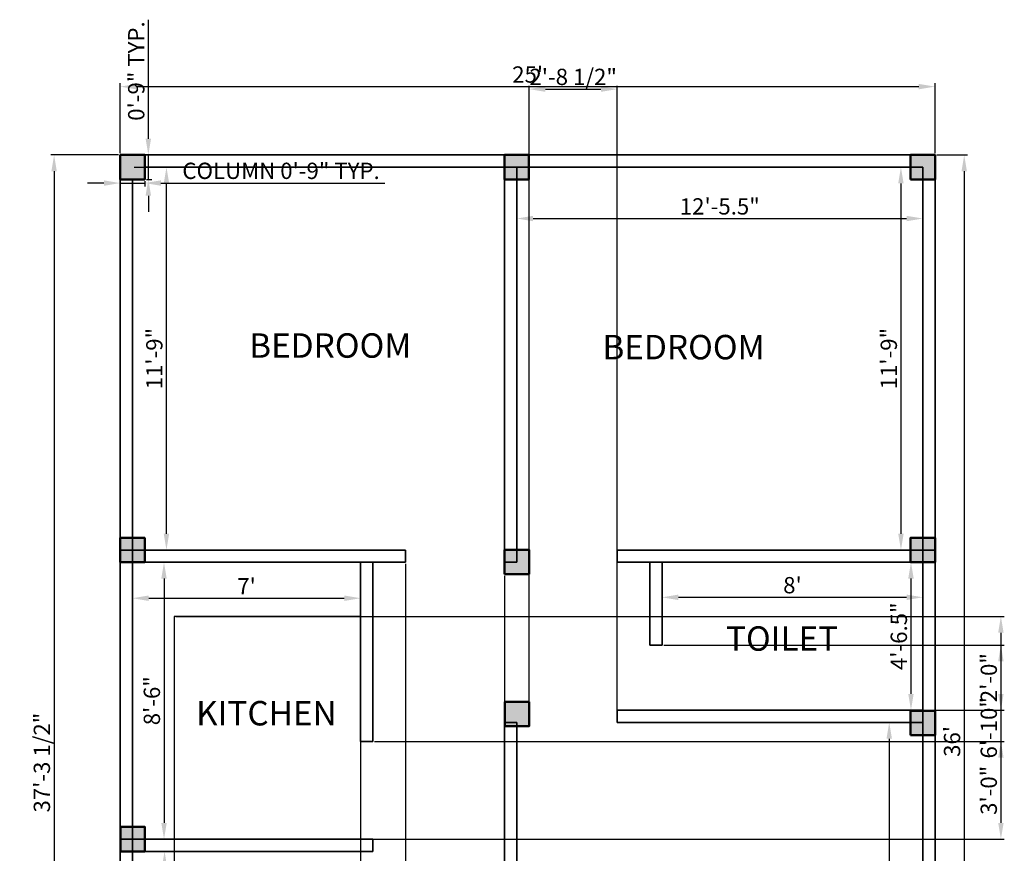
# Model space of a CAD drawing. Units: inches. Extents: x 6892 to 7255, y 6029 to 6556.
# Tile 2 of 2: x 6892 to 7255, y 6249 to 6556. Entities that reach past the tile are written whole.
import ezdxf

# ---------------------------------------------------------------- set-up
doc = ezdxf.new("R2010")
doc.units = ezdxf.units.IN
for name, color, linetype, lineweight in [('A-ANNO-DIMS', 2, 'Continuous', 18), ('A-AREA-IDEN', 7, 'Continuous', 25), ('A-COLS', 7, 'Continuous', 50), ('A-COLS-PATT', 1, 'Continuous', 13), ('A-FLOR-FIXT', 8, 'Continuous', 25), ('A-WALL', 7, 'Continuous', 35)]:
    doc.layers.add(name, color=color, linetype=linetype, lineweight=lineweight)
doc.styles.get("Standard").update_dxf_attribs({"font": 'arial.ttf'})
doc.dimstyles.new('ISO-25', dxfattribs={"dimtxt": 6, "dimasz": 6, "dimexe": 1.25, "dimexo": 0.625, "dimtad": 1, "dimlunit": 3, "dimtxsty": 'Standard', "dimcen": 2.5, "dimadec": 0, "dimazin": 0, "dimtfac": 1, "dimtmove": 0, "dimatfit": 3, "dimfxl": 1, "dimarcsym": 0})

# ---------------------------------------------------------------- blocks, each defined once
blk = doc.blocks.new('*D1')
at = {"layer": 'A-ANNO-DIMS', "color": 0, "lineweight": -2, "transparency": 16777216}
for p, q in [((6945.77, 6249.77), (6946.64, 6249.77)), ((6945.39, 6084.77), (6945.39, 6243.77)), ((6945.77, 6078.77), (6946.64, 6078.77))]:
    blk.add_line(p, q, dxfattribs=at)
at = {"layer": 'A-ANNO-DIMS', "color": 0, "transparency": 16777216}
for points in [[(6944.39, 6243.77), (6946.39, 6243.77), (6945.39, 6249.77)], [(6944.39, 6084.77), (6946.39, 6084.77), (6945.39, 6078.77)]]:
    blk.add_solid(points, dxfattribs=at)
at = {"layer": 'Defpoints', "color": 0, "transparency": 16777216}
for p in [(6945.15, 6249.77), (6945.39, 6249.77), (6945.15, 6078.77)]:
    blk.add_point(p, dxfattribs=at)
at = {"layer": 'A-ANNO-DIMS', "color": 0, "transparency": 16777216, "insert": (6941.7, 6164.27), "char_height": 6, "attachment_point": 5, "rotation": 90}
blk.add_mtext('14\'-3"', dxfattribs=at)
blk = doc.blocks.new('*D3')
at = {"layer": 'A-ANNO-DIMS', "color": 0, "lineweight": -2, "transparency": 16777216}
for p, q in [((6933.57, 6355.65), (6933.57, 6341.77)), ((7017.57, 6355.65), (7017.57, 6341.77)), ((6939.57, 6343.02), (7011.57, 6343.02))]:
    blk.add_line(p, q, dxfattribs=at)
at = {"layer": 'A-ANNO-DIMS', "color": 0, "transparency": 16777216}
for points in [[(6939.57, 6344.02), (6939.57, 6342.02), (6933.57, 6343.02)], [(7011.57, 6344.02), (7011.57, 6342.02), (7017.57, 6343.02)]]:
    blk.add_solid(points, dxfattribs=at)
at = {"layer": 'Defpoints', "color": 0, "transparency": 16777216}
for p in [(6933.57, 6356.27), (7017.57, 6356.27), (7017.57, 6343.02)]:
    blk.add_point(p, dxfattribs=at)
at = {"layer": 'A-ANNO-DIMS', "color": 0, "transparency": 16777216, "insert": (6975.57, 6346.64), "char_height": 6, "attachment_point": 5}
blk.add_mtext("7'", dxfattribs=at)
blk = doc.blocks.new('*D4')
at = {"layer": 'A-ANNO-DIMS', "color": 0, "lineweight": -2, "transparency": 16777216}
for p, q in [((6934.2, 6356.27), (6946.44, 6356.27)), ((6945.19, 6350.27), (6945.19, 6260.27)), ((6934.2, 6254.27), (6946.44, 6254.27))]:
    blk.add_line(p, q, dxfattribs=at)
at = {"layer": 'A-ANNO-DIMS', "color": 0, "transparency": 16777216}
for points in [[(6944.19, 6350.27), (6946.19, 6350.27), (6945.19, 6356.27)], [(6944.19, 6260.27), (6946.19, 6260.27), (6945.19, 6254.27)]]:
    blk.add_solid(points, dxfattribs=at)
at = {"layer": 'Defpoints', "color": 0, "transparency": 16777216}
for p in [(6933.57, 6356.27), (6933.57, 6254.27), (6945.19, 6254.27)]:
    blk.add_point(p, dxfattribs=at)
at = {"layer": 'A-ANNO-DIMS', "color": 0, "transparency": 16777216, "insert": (6941.5, 6305.27), "char_height": 6, "attachment_point": 5, "rotation": 90}
blk.add_mtext('8\'-6"', dxfattribs=at)
blk = doc.blocks.new('*D5')
at = {"layer": 'A-ANNO-DIMS', "color": 0, "lineweight": -2, "transparency": 16777216}
for p, q in [((6934.2, 6501.77), (6947.34, 6501.77)), ((6946.09, 6366.77), (6946.09, 6495.77)), ((6934.2, 6360.77), (6947.34, 6360.77))]:
    blk.add_line(p, q, dxfattribs=at)
at = {"layer": 'A-ANNO-DIMS', "color": 0, "transparency": 16777216}
for points in [[(6945.09, 6495.77), (6947.09, 6495.77), (6946.09, 6501.77)], [(6945.09, 6366.77), (6947.09, 6366.77), (6946.09, 6360.77)]]:
    blk.add_solid(points, dxfattribs=at)
at = {"layer": 'Defpoints', "color": 0, "transparency": 16777216}
for p in [(6933.57, 6501.77), (6946.09, 6501.77), (6933.57, 6360.77)]:
    blk.add_point(p, dxfattribs=at)
at = {"layer": 'A-ANNO-DIMS', "color": 0, "transparency": 16777216, "insert": (6942.4, 6431.27), "char_height": 6, "attachment_point": 5, "rotation": 90}
blk.add_mtext('11\'-9"', dxfattribs=at)
blk = doc.blocks.new('*D6')
at = {"layer": 'A-ANNO-DIMS', "color": 0, "lineweight": -2, "transparency": 16777216}
for p, q in [((7075.07, 6501.15), (7075.07, 6481.61)), ((7224.57, 6501.15), (7224.57, 6481.61)), ((7081.07, 6482.86), (7218.57, 6482.86))]:
    blk.add_line(p, q, dxfattribs=at)
at = {"layer": 'A-ANNO-DIMS', "color": 0, "transparency": 16777216}
for points in [[(7081.07, 6483.86), (7081.07, 6481.86), (7075.07, 6482.86)], [(7218.57, 6483.86), (7218.57, 6481.86), (7224.57, 6482.86)]]:
    blk.add_solid(points, dxfattribs=at)
at = {"layer": 'Defpoints', "color": 0, "transparency": 16777216}
for p in [(7075.07, 6501.77), (7224.57, 6501.77), (7224.57, 6482.86)]:
    blk.add_point(p, dxfattribs=at)
at = {"layer": 'A-ANNO-DIMS', "color": 0, "transparency": 16777216, "insert": (7149.82, 6486.55), "char_height": 6, "attachment_point": 5}
blk.add_mtext('12\'-5.5"', dxfattribs=at)
blk = doc.blocks.new('*D7')
at = {"layer": 'A-ANNO-DIMS', "color": 0, "lineweight": -2, "transparency": 16777216}
for p, q in [((7223.95, 6501.77), (7215.26, 6501.77)), ((7216.51, 6495.77), (7216.51, 6366.77)), ((7223.95, 6360.77), (7215.26, 6360.77))]:
    blk.add_line(p, q, dxfattribs=at)
at = {"layer": 'A-ANNO-DIMS', "color": 0, "transparency": 16777216}
for points in [[(7215.51, 6495.77), (7217.51, 6495.77), (7216.51, 6501.77)], [(7215.51, 6366.77), (7217.51, 6366.77), (7216.51, 6360.77)]]:
    blk.add_solid(points, dxfattribs=at)
at = {"layer": 'Defpoints', "color": 0, "transparency": 16777216}
for p in [(7224.57, 6501.77), (7216.51, 6360.77), (7224.57, 6360.77)]:
    blk.add_point(p, dxfattribs=at)
at = {"layer": 'A-ANNO-DIMS', "color": 0, "transparency": 16777216, "insert": (7212.82, 6431.27), "char_height": 6, "attachment_point": 5, "rotation": 90}
blk.add_mtext('11\'-9"', dxfattribs=at)
blk = doc.blocks.new('*D8')
at = {"layer": 'A-ANNO-DIMS', "color": 0, "lineweight": -2, "transparency": 16777216}
for p, q in [((7128.57, 6355.65), (7128.57, 6342.1)), ((7224.57, 6355.65), (7224.57, 6342.1)), ((7134.57, 6343.35), (7218.57, 6343.35))]:
    blk.add_line(p, q, dxfattribs=at)
at = {"layer": 'A-ANNO-DIMS', "color": 0, "transparency": 16777216}
for points in [[(7134.57, 6344.35), (7134.57, 6342.35), (7128.57, 6343.35)], [(7218.57, 6344.35), (7218.57, 6342.35), (7224.57, 6343.35)]]:
    blk.add_solid(points, dxfattribs=at)
at = {"layer": 'Defpoints', "color": 0, "transparency": 16777216}
for p in [(7128.57, 6356.27), (7224.57, 6356.27), (7224.57, 6343.35)]:
    blk.add_point(p, dxfattribs=at)
at = {"layer": 'A-ANNO-DIMS', "color": 0, "transparency": 16777216, "insert": (7176.57, 6347.04), "char_height": 6, "attachment_point": 5}
blk.add_mtext("8'", dxfattribs=at)
blk = doc.blocks.new('*D9')
at = {"layer": 'A-ANNO-DIMS', "color": 0, "lineweight": -2, "transparency": 16777216}
for p, q in [((7223.95, 6356.27), (7218.96, 6356.27)), ((7220.21, 6350.27), (7220.21, 6307.77)), ((7223.95, 6301.77), (7218.96, 6301.77))]:
    blk.add_line(p, q, dxfattribs=at)
at = {"layer": 'A-ANNO-DIMS', "color": 0, "transparency": 16777216}
for points in [[(7219.21, 6350.27), (7221.21, 6350.27), (7220.21, 6356.27)], [(7219.21, 6307.77), (7221.21, 6307.77), (7220.21, 6301.77)]]:
    blk.add_solid(points, dxfattribs=at)
at = {"layer": 'Defpoints', "color": 0, "transparency": 16777216}
for p in [(7224.57, 6356.27), (7220.21, 6301.77), (7224.57, 6301.77)]:
    blk.add_point(p, dxfattribs=at)
at = {"layer": 'A-ANNO-DIMS', "color": 0, "transparency": 16777216, "insert": (7216.52, 6329.02), "char_height": 6, "attachment_point": 5, "rotation": 90}
blk.add_mtext('4\'-6.5"', dxfattribs=at)
blk = doc.blocks.new('*D11')
at = {"layer": 'A-ANNO-DIMS', "color": 0, "lineweight": -2, "transparency": 16777216}
for p, q in [((7223.95, 6297.27), (7210.95, 6297.27)), ((7212.2, 6291.27), (7212.2, 6167.27)), ((7223.95, 6161.27), (7210.95, 6161.27))]:
    blk.add_line(p, q, dxfattribs=at)
at = {"layer": 'A-ANNO-DIMS', "color": 0, "transparency": 16777216}
for points in [[(7211.2, 6291.27), (7213.2, 6291.27), (7212.2, 6297.27)], [(7211.2, 6167.27), (7213.2, 6167.27), (7212.2, 6161.27)]]:
    blk.add_solid(points, dxfattribs=at)
at = {"layer": 'Defpoints', "color": 0, "transparency": 16777216}
for p in [(7224.57, 6297.27), (7212.2, 6161.27), (7224.57, 6161.27)]:
    blk.add_point(p, dxfattribs=at)
at = {"layer": 'A-ANNO-DIMS', "color": 0, "transparency": 16777216, "insert": (7208.56, 6229.27), "char_height": 6, "attachment_point": 5, "rotation": 90}
blk.add_mtext('11\'-4"', dxfattribs=at)
blk = doc.blocks.new('*D15')
at = {"layer": 'A-ANNO-DIMS', "color": 0, "lineweight": -2, "transparency": 16777216}
for p, q in [((6929.07, 6506.9), (6929.07, 6532.69)), ((7229.07, 6506.9), (7229.07, 6532.69)), ((6935.07, 6531.44), (7223.07, 6531.44))]:
    blk.add_line(p, q, dxfattribs=at)
at = {"layer": 'A-ANNO-DIMS', "color": 0, "transparency": 16777216}
for points in [[(6935.07, 6532.44), (6935.07, 6530.44), (6929.07, 6531.44)], [(7223.07, 6532.44), (7223.07, 6530.44), (7229.07, 6531.44)]]:
    blk.add_solid(points, dxfattribs=at)
at = {"layer": 'Defpoints', "color": 0, "transparency": 16777216}
for p in [(7229.07, 6531.44), (6929.07, 6506.27), (7229.07, 6506.27)]:
    blk.add_point(p, dxfattribs=at)
at = {"layer": 'A-ANNO-DIMS', "color": 0, "transparency": 16777216, "insert": (7079.07, 6535.12), "char_height": 6, "attachment_point": 5}
blk.add_mtext("25'", dxfattribs=at)
blk = doc.blocks.new('*D16')
at = {"layer": 'A-ANNO-DIMS', "color": 0, "lineweight": -2, "transparency": 16777216}
for p, q in [((7229.7, 6506.27), (7241.06, 6506.27)), ((7239.81, 6500.27), (7239.81, 6080.27)), ((7229.7, 6074.27), (7241.06, 6074.27))]:
    blk.add_line(p, q, dxfattribs=at)
at = {"layer": 'A-ANNO-DIMS', "color": 0, "transparency": 16777216}
for points in [[(7238.81, 6500.27), (7240.81, 6500.27), (7239.81, 6506.27)], [(7238.81, 6080.27), (7240.81, 6080.27), (7239.81, 6074.27)]]:
    blk.add_solid(points, dxfattribs=at)
at = {"layer": 'Defpoints', "color": 0, "transparency": 16777216}
for p in [(7229.07, 6506.27), (7229.07, 6074.27), (7239.81, 6074.27)]:
    blk.add_point(p, dxfattribs=at)
at = {"layer": 'A-ANNO-DIMS', "color": 0, "transparency": 16777216, "insert": (7236.12, 6290.27), "char_height": 6, "attachment_point": 5, "rotation": 90}
blk.add_mtext("36'", dxfattribs=at)
blk = doc.blocks.new('COL-9IN-SQ')
blk.add_lwpolyline([(0, 0), (9, 0), (9, 9), (0, 9)], close=True)
blk = doc.blocks.new('*D18')
at = {"layer": 'A-ANNO-DIMS', "color": 0, "lineweight": -2, "transparency": 16777216}
for p, q in [((6929.07, 6496.65), (6929.07, 6494.67)), ((6938.07, 6496.65), (6938.07, 6494.67)), ((6923.07, 6495.92), (6917.07, 6495.92)), ((6929.07, 6495.92), (6938.07, 6495.92)), ((6944.07, 6495.92), (7026.48, 6495.92))]:
    blk.add_line(p, q, dxfattribs=at)
at = {"layer": 'A-ANNO-DIMS', "color": 0, "transparency": 16777216}
for points in [[(6923.07, 6496.92), (6923.07, 6494.92), (6929.07, 6495.92)], [(6944.07, 6496.92), (6944.07, 6494.92), (6938.07, 6495.92)]]:
    blk.add_solid(points, dxfattribs=at)
at = {"layer": 'Defpoints', "color": 0, "transparency": 16777216}
for p in [(6929.07, 6497.27), (6938.07, 6497.27), (6938.07, 6495.92)]:
    blk.add_point(p, dxfattribs=at)
at = {"layer": 'A-ANNO-DIMS', "color": 0, "transparency": 16777216, "insert": (6988.28, 6499.65), "char_height": 6, "attachment_point": 5}
blk.add_mtext('COLUMN 0\'-9" TYP.', dxfattribs=at)
blk = doc.blocks.new('*D19')
at = {"layer": 'A-ANNO-DIMS', "color": 0, "lineweight": -2, "transparency": 16777216}
for p, q in [((6939.42, 6512.27), (6939.42, 6556.09)), ((6938.7, 6506.27), (6940.67, 6506.27)), ((6939.42, 6497.27), (6939.42, 6506.27)), ((6938.7, 6497.27), (6940.67, 6497.27)), ((6939.42, 6491.27), (6939.42, 6485.27))]:
    blk.add_line(p, q, dxfattribs=at)
at = {"layer": 'A-ANNO-DIMS', "color": 0, "transparency": 16777216}
for points in [[(6938.42, 6512.27), (6940.42, 6512.27), (6939.42, 6506.27)], [(6938.42, 6491.27), (6940.42, 6491.27), (6939.42, 6497.27)]]:
    blk.add_solid(points, dxfattribs=at)
at = {"layer": 'Defpoints', "color": 0, "transparency": 16777216}
for p in [(6938.07, 6506.27), (6939.42, 6506.27), (6938.07, 6497.27)]:
    blk.add_point(p, dxfattribs=at)
at = {"layer": 'A-ANNO-DIMS', "color": 0, "transparency": 16777216, "insert": (6935.74, 6537.18), "char_height": 6, "attachment_point": 5, "rotation": 90}
blk.add_mtext('0\'-9" TYP.', dxfattribs=at)
blk = doc.blocks.new('*D20')
at = {"layer": 'A-ANNO-DIMS', "color": 0, "lineweight": -2, "transparency": 16777216}
for p, q in [((6928.45, 6506.27), (6903.48, 6506.27)), ((6904.73, 6500.27), (6904.73, 6064.66)), ((7017.45, 6058.66), (6903.48, 6058.66))]:
    blk.add_line(p, q, dxfattribs=at)
at = {"layer": 'A-ANNO-DIMS', "color": 0, "transparency": 16777216}
for points in [[(6903.73, 6500.27), (6905.73, 6500.27), (6904.73, 6506.27)], [(6903.73, 6064.66), (6905.73, 6064.66), (6904.73, 6058.66)]]:
    blk.add_solid(points, dxfattribs=at)
at = {"layer": 'Defpoints', "color": 0, "transparency": 16777216}
for p in [(6929.07, 6506.27), (6904.73, 6058.66), (7018.07, 6058.66)]:
    blk.add_point(p, dxfattribs=at)
at = {"layer": 'A-ANNO-DIMS', "color": 0, "transparency": 16777216, "insert": (6901, 6282.47), "char_height": 6, "attachment_point": 5, "rotation": 90}
blk.add_mtext('37\'-3 1/2"', dxfattribs=at)
blk = doc.blocks.new('*D22')
at = {"layer": 'A-ANNO-DIMS', "color": 0, "lineweight": -2, "transparency": 16777216}
for p, q in [((7034.07, 6355.65), (7034.07, 6033.16)), ((7070.6, 6351.27), (7070.6, 6033.16)), ((7040.07, 6034.41), (7064.6, 6034.41))]:
    blk.add_line(p, q, dxfattribs=at)
at = {"layer": 'A-ANNO-DIMS', "color": 0, "transparency": 16777216}
for points in [[(7040.07, 6035.41), (7040.07, 6033.41), (7034.07, 6034.41)], [(7064.6, 6035.41), (7064.6, 6033.41), (7070.6, 6034.41)]]:
    blk.add_solid(points, dxfattribs=at)
at = {"layer": 'Defpoints', "color": 0, "transparency": 16777216}
for p in [(7034.07, 6356.27), (7070.6, 6351.9), (7070.6, 6034.41)]:
    blk.add_point(p, dxfattribs=at)
at = {"layer": 'A-ANNO-DIMS', "color": 0, "transparency": 16777216, "insert": (7052.34, 6038.14), "char_height": 6, "attachment_point": 5}
blk.add_mtext('3\'-0 1/2"', dxfattribs=at)
blk = doc.blocks.new('*D23')
at = {"layer": 'A-ANNO-DIMS', "color": 0, "lineweight": -2, "transparency": 16777216}
for p, q in [((7079.6, 6361.52), (7079.6, 6531.77)), ((7085.6, 6530.52), (7106.07, 6530.52)), ((7112.07, 6361.4), (7112.07, 6531.77))]:
    blk.add_line(p, q, dxfattribs=at)
at = {"layer": 'A-ANNO-DIMS', "color": 0, "transparency": 16777216}
for points in [[(7085.6, 6531.52), (7085.6, 6529.52), (7079.6, 6530.52)], [(7106.07, 6531.52), (7106.07, 6529.52), (7112.07, 6530.52)]]:
    blk.add_solid(points, dxfattribs=at)
at = {"layer": 'Defpoints', "color": 0, "transparency": 16777216}
for p in [(7112.07, 6530.52), (7079.6, 6360.9), (7112.07, 6360.77)]:
    blk.add_point(p, dxfattribs=at)
at = {"layer": 'A-ANNO-DIMS', "color": 0, "transparency": 16777216, "insert": (7095.84, 6534.25), "char_height": 6, "attachment_point": 5}
blk.add_mtext('2\'-8 1/2"', dxfattribs=at)
blk = doc.blocks.new('*D24')
at = {"layer": 'A-ANNO-DIMS', "color": 0, "lineweight": -2, "transparency": 16777216}
for p, q in [((7022.7, 6290.27), (7254.57, 6290.27)), ((7253.32, 6284.27), (7253.32, 6260.27)), ((7022.7, 6254.27), (7254.57, 6254.27))]:
    blk.add_line(p, q, dxfattribs=at)
at = {"layer": 'A-ANNO-DIMS', "color": 0, "transparency": 16777216}
for points in [[(7252.32, 6284.27), (7254.32, 6284.27), (7253.32, 6290.27)], [(7252.32, 6260.27), (7254.32, 6260.27), (7253.32, 6254.27)]]:
    blk.add_solid(points, dxfattribs=at)
at = {"layer": 'Defpoints', "color": 0, "transparency": 16777216}
for p in [(7022.07, 6290.27), (7022.07, 6254.27), (7253.32, 6254.27)]:
    blk.add_point(p, dxfattribs=at)
at = {"layer": 'A-ANNO-DIMS', "color": 0, "transparency": 16777216, "insert": (7249.63, 6272.27), "char_height": 6, "attachment_point": 5, "rotation": 90}
blk.add_mtext('3\'-0"', dxfattribs=at)
blk = doc.blocks.new('*D25')
at = {"layer": 'A-ANNO-DIMS', "color": 0, "lineweight": -2, "transparency": 16777216}
for p, q in [((7129.2, 6325.77), (7254.57, 6325.77)), ((7253.32, 6319.77), (7253.32, 6307.77)), ((7112.7, 6301.77), (7254.57, 6301.77))]:
    blk.add_line(p, q, dxfattribs=at)
at = {"layer": 'A-ANNO-DIMS', "color": 0, "transparency": 16777216}
for points in [[(7252.32, 6319.77), (7254.32, 6319.77), (7253.32, 6325.77)], [(7252.32, 6307.77), (7254.32, 6307.77), (7253.32, 6301.77)]]:
    blk.add_solid(points, dxfattribs=at)
at = {"layer": 'Defpoints', "color": 0, "transparency": 16777216}
for p in [(7128.57, 6325.77), (7112.07, 6301.77), (7253.32, 6301.77)]:
    blk.add_point(p, dxfattribs=at)
at = {"layer": 'A-ANNO-DIMS', "color": 0, "transparency": 16777216, "insert": (7249.64, 6313.77), "char_height": 6, "attachment_point": 5, "rotation": 90}
blk.add_mtext('2\'-0"', dxfattribs=at)
blk = doc.blocks.new('*D26')
at = {"layer": 'A-ANNO-DIMS', "color": 0, "lineweight": -2, "transparency": 16777216}
for p, q in [((7079.63, 6296.47), (7079.63, 6531.77)), ((7085.63, 6530.52), (7106.07, 6530.52)), ((7112.07, 6297.9), (7112.07, 6531.77))]:
    blk.add_line(p, q, dxfattribs=at)
at = {"layer": 'A-ANNO-DIMS', "color": 0, "transparency": 16777216}
for points in [[(7085.63, 6531.52), (7085.63, 6529.52), (7079.63, 6530.52)], [(7106.07, 6531.52), (7106.07, 6529.52), (7112.07, 6530.52)]]:
    blk.add_solid(points, dxfattribs=at)
at = {"layer": 'Defpoints', "color": 0, "transparency": 16777216}
for p in [(7112.07, 6530.52), (7112.07, 6297.27), (7079.63, 6295.85)]:
    blk.add_point(p, dxfattribs=at)
at = {"layer": 'A-ANNO-DIMS', "color": 0, "transparency": 16777216, "insert": (7095.85, 6534.25), "char_height": 6, "attachment_point": 5}
blk.add_mtext('2\'-8 1/2"', dxfattribs=at)
blk = doc.blocks.new('*D28')
at = {"layer": 'A-ANNO-DIMS', "color": 0, "lineweight": -2, "transparency": 16777216}
for p, q in [((6948.94, 6335.71), (6948.94, 6033.16)), ((7017.57, 6335.71), (7017.57, 6033.16)), ((6954.94, 6034.41), (7011.57, 6034.41))]:
    blk.add_line(p, q, dxfattribs=at)
at = {"layer": 'A-ANNO-DIMS', "color": 0, "transparency": 16777216}
for points in [[(6954.94, 6035.41), (6954.94, 6033.41), (6948.94, 6034.41)], [(7011.57, 6035.41), (7011.57, 6033.41), (7017.57, 6034.41)]]:
    blk.add_solid(points, dxfattribs=at)
at = {"layer": 'Defpoints', "color": 0, "transparency": 16777216}
for p in [(6948.94, 6336.33), (7017.57, 6336.33), (7017.57, 6034.41)]:
    blk.add_point(p, dxfattribs=at)
at = {"layer": 'A-ANNO-DIMS', "color": 0, "transparency": 16777216, "insert": (6983.26, 6038.14), "char_height": 6, "attachment_point": 5}
blk.add_mtext('5\'-8 1/2"', dxfattribs=at)
blk = doc.blocks.new('*D29')
at = {"layer": 'A-ANNO-DIMS', "color": 0, "lineweight": -2, "transparency": 16777216}
for p, q in [((6949.57, 6336.33), (7254.57, 6336.33)), ((7253.32, 6330.33), (7253.32, 6260.27)), ((6949.57, 6254.27), (7254.57, 6254.27))]:
    blk.add_line(p, q, dxfattribs=at)
at = {"layer": 'A-ANNO-DIMS', "color": 0, "transparency": 16777216}
for points in [[(7252.32, 6330.33), (7254.32, 6330.33), (7253.32, 6336.33)], [(7252.32, 6260.27), (7254.32, 6260.27), (7253.32, 6254.27)]]:
    blk.add_solid(points, dxfattribs=at)
at = {"layer": 'Defpoints', "color": 0, "transparency": 16777216}
for p in [(6948.94, 6336.33), (6948.94, 6254.27), (7253.32, 6254.27)]:
    blk.add_point(p, dxfattribs=at)
at = {"layer": 'A-ANNO-DIMS', "color": 0, "transparency": 16777216, "insert": (7249.64, 6295.3), "char_height": 6, "attachment_point": 5, "rotation": 90}
blk.add_mtext('6\'-10"', dxfattribs=at)

msp = doc.modelspace()

# ---------------------------------------------------------------- hatches: boundary and pattern name
at = {"layer": 'A-COLS-PATT'}
h = msp.add_hatch(color=256, dxfattribs=at)
h.dxf.hatch_style = 1
h.paths.add_polyline_path([(6938.074, 6506.271), (6929.074, 6506.271), (6929.074, 6497.271), (6938.074, 6497.271)])
h.paths.add_polyline_path([(7079.574, 6506.271), (7070.574, 6506.271), (7070.574, 6501.771), (7079.574, 6501.771)])
h.paths.add_polyline_path([(7079.574, 6501.771), (7075.074, 6501.771), (7075.074, 6497.271), (7079.574, 6497.271)])
h.paths.add_polyline_path([(7075.074, 6501.771), (7070.574, 6501.771), (7070.574, 6497.271), (7075.074, 6497.271)])
h.paths.add_polyline_path([(7229.074, 6506.271), (7220.074, 6506.271), (7220.074, 6501.771), (7224.574, 6501.771), (7224.574, 6497.271), (7229.074, 6497.271)])
h.paths.add_polyline_path([(7224.574, 6501.771), (7220.074, 6501.771), (7220.074, 6497.271), (7224.574, 6497.271)], flags=17)
h.paths.add_polyline_path([(7224.574, 6365.271), (7220.074, 6365.271), (7220.074, 6360.771), (7224.574, 6360.771)])
h.paths.add_polyline_path([(7229.074, 6365.271), (7224.574, 6365.271), (7224.574, 6360.771), (7229.074, 6360.771)])
h.paths.add_polyline_path([(7229.074, 6360.771), (7224.574, 6360.771), (7224.574, 6356.271), (7229.074, 6356.271)])
h.paths.add_polyline_path([(7224.574, 6360.771), (7220.074, 6360.771), (7220.074, 6356.271), (7224.574, 6356.271)])
h.paths.add_polyline_path([(6938.094, 6360.771), (6933.574, 6360.771), (6933.574, 6356.271), (6938.094, 6356.271)])
h.paths.add_polyline_path([(6938.094, 6365.243), (6933.574, 6365.243), (6933.574, 6360.771), (6938.094, 6360.771)])
h.paths.add_polyline_path([(6933.574, 6365.243), (6929.094, 6365.243), (6929.094, 6360.771), (6933.574, 6360.771)])
h.paths.add_polyline_path([(6933.574, 6360.771), (6929.094, 6360.771), (6929.094, 6356.271), (6933.574, 6356.271)])
h.paths.add_polyline_path([(7075.074, 6360.771), (7070.605, 6360.771), (7070.605, 6356.271), (7075.074, 6356.271)], flags=17)
h.paths.add_polyline_path([(7079.605, 6360.898), (7075.074, 6360.898), (7075.074, 6356.271), (7070.605, 6356.271), (7070.605, 6351.898), (7079.605, 6351.898)])
h.paths.add_polyline_path([(7079.634, 6304.845), (7070.634, 6304.845), (7070.634, 6297.271), (7075.074, 6297.271), (7075.074, 6295.845), (7079.634, 6295.845)])
h.paths.add_polyline_path([(7075.074, 6297.271), (7070.634, 6297.271), (7070.634, 6295.845), (7075.074, 6295.845)], flags=17)
h.paths.add_polyline_path([(6938.172, 6258.771), (6933.574, 6258.771), (6933.574, 6254.271), (6938.172, 6254.271)])
h.paths.add_polyline_path([(6933.574, 6258.771), (6929.172, 6258.771), (6929.172, 6254.271), (6933.574, 6254.271)])
h.paths.add_polyline_path([(6933.574, 6254.271), (6929.172, 6254.271), (6929.172, 6249.771), (6933.574, 6249.771)])
h.paths.add_polyline_path([(6938.172, 6254.271), (6933.574, 6254.271), (6933.574, 6249.771), (6938.172, 6249.771)])
h.paths.add_polyline_path([(7229.074, 6301.605), (7224.574, 6301.605), (7224.574, 6297.271), (7224.574, 6292.605), (7229.074, 6292.605)])
h.paths.add_polyline_path([(7224.574, 6297.271), (7220.074, 6297.271), (7220.074, 6292.605), (7224.574, 6292.605)])
h.paths.add_polyline_path([(7224.574, 6301.605), (7220.074, 6301.605), (7220.074, 6297.271), (7224.574, 6297.271)])

# ---------------------------------------------------------------- linework, layer by layer
at = {"layer": 'A-FLOR-FIXT'}
for p, q in [((7017.574, 6336.334), (6948.942, 6336.334)), ((6948.942, 6336.334), (6948.942, 6254.271))]:
    msp.add_line(p, q, dxfattribs=at)
at = {"layer": 'A-WALL'}
for p, q in [((6929.074, 6506.271), (7229.074, 6506.271)), ((6929.074, 6074.271), (6929.074, 6506.271)), ((7229.074, 6506.271), (7229.074, 6074.271)), ((6938.074, 6501.771), (7224.574, 6501.771)), ((7070.574, 6501.771), (7070.574, 6356.271)), ((7075.074, 6501.771), (7075.074, 6356.271)), ((7224.574, 6501.771), (7224.574, 6074.271)), ((6933.574, 6074.271), (6933.574, 6497.271)), ((7034.074, 6360.771), (6929.074, 6360.771)), ((7034.074, 6356.271), (7034.074, 6360.771)), ((7075.074, 6360.771), (7070.574, 6360.771)), ((7229.074, 6360.771), (7112.074, 6360.771)), ((7112.074, 6356.271), (7112.074, 6360.771)), ((7034.074, 6356.271), (6929.074, 6356.271)), ((7017.574, 6356.271), (7017.574, 6290.271)), ((7022.074, 6356.271), (7022.074, 6290.271)), ((7022.074, 6356.271), (7034.074, 6356.271)), ((7075.074, 6356.271), (7070.574, 6356.271)), ((7229.074, 6356.271), (7112.074, 6356.271)), ((7124.074, 6356.271), (7112.074, 6356.271)), ((7124.074, 6356.271), (7124.074, 6325.771)), ((7128.574, 6356.271), (7128.574, 6325.771)), ((7224.574, 6356.271), (7224.574, 6297.271)), ((7124.074, 6325.771), (7128.574, 6325.771)), ((7112.074, 6301.771), (7224.574, 6301.771)), ((7112.074, 6301.771), (7112.074, 6297.271)), ((7075.074, 6297.271), (7070.574, 6297.271)), ((7070.574, 6297.271), (7070.574, 6249.771)), ((7075.074, 6249.771), (7075.074, 6297.271)), ((7112.074, 6297.271), (7224.574, 6297.271)), ((7017.574, 6290.271), (7022.074, 6290.271)), ((7022.074, 6254.271), (6929.074, 6254.271)), ((7022.074, 6254.271), (7022.074, 6249.771)), ((7022.074, 6249.771), (6929.074, 6249.771)), ((7070.574, 6249.771), (7070.574, 6156.771)), ((7075.074, 6249.771), (7075.074, 6156.771))]:
    msp.add_line(p, q, dxfattribs=at)

# ---------------------------------------------------------------- block references
at = {"layer": 'A-COLS'}
for p in [(6929.074, 6497.271), (7070.574, 6497.271), (7220.074, 6497.271), (6929.095, 6356.243), (7220.074, 6356.271), (7070.605, 6351.897), (7070.634, 6295.845), (7220.074, 6292.604), (6929.172, 6249.771)]:
    msp.add_blockref('COL-9IN-SQ', p, dxfattribs=at)

# ---------------------------------------------------------------- texts
at = {"layer": 'A-AREA-IDEN', "char_height": 9, "attachment_point": 1}
for s, width, heights, insert in [('BEDROOM', 37.83075, [0], (6976.54, 6440.588)), ('BEDROOM', 43.8085, [0.785], (7106.616, 6439.999)), ('TOILET', 37.75614, [0], (7152.097, 6332.674)), ('KITCHEN', 42.3338, [0], (6957.012, 6305.161))]:
    msp.add_mtext_dynamic_manual_height_columns(s, width=width, gutter_width=12.5, heights=heights, dxfattribs=dict(at, insert=insert))

# ---------------------------------------------------------------- dimensions: what is measured, and where the dimension line sits
at = {"layer": 'A-ANNO-DIMS'}
dim = msp.add_linear_dim(base=(6939.424, 6506.271), p1=(6938.074, 6497.271), p2=(6938.074, 6506.271), angle=90, text='<> TYP.', dimstyle='ISO-25', override={"dimdec": 1, "dimlfac": 1, "dimrnd": 0, "dimzin": 1, "dimdsep": 46, "dimlunit": 4, "dimfrac": 2}, dxfattribs=at)
dim.commit()
dim.dimension.update_dxf_attribs({"geometry": '*D19', "text_midpoint": (6935.735, 6537.183)})
for base, p1, p2, override, picture, middle in [((7112.074, 6530.521), (7079.605, 6360.898), (7112.074, 6360.771), {"dimdec": 1, "dimlfac": 1, "dimrnd": 0, "dimzin": 1, "dimdsep": 46, "dimlunit": 4, "dimfrac": 2}, '*D23', (7095.839, 6534.249)), ((7112.074, 6530.521), (7079.634, 6295.845), (7112.074, 6297.271), {"dimdec": 1, "dimlfac": 1, "dimrnd": 0, "dimzin": 1, "dimdsep": 46, "dimlunit": 4, "dimfrac": 2}, '*D26', (7095.854, 6534.249)), ((7229.074, 6531.436), (6929.074, 6506.271), (7229.074, 6506.271), {"dimclrd": 0, "dimclre": 0, "dimclrt": 0}, '*D15', (7079.074, 6535.125)), ((7224.574, 6482.864), (7075.074, 6501.771), (7224.574, 6501.771), {"dimclrd": 0, "dimclre": 0, "dimclrt": 0}, '*D6', (7149.824, 6486.553)), ((7017.574, 6343.019), (6933.574, 6356.271), (7017.574, 6356.271), {"dimclrd": 0, "dimclre": 0, "dimclrt": 0}, '*D3', (6975.574, 6346.644)), ((7070.605, 6034.411), (7034.074, 6356.271), (7070.605, 6351.898), {"dimdec": 1, "dimlfac": 1, "dimrnd": 0, "dimzin": 1, "dimdsep": 46, "dimlunit": 4, "dimfrac": 2}, '*D22', (7052.339, 6038.14)), ((7224.574, 6343.349), (7128.574, 6356.271), (7224.574, 6356.271), {"dimclrd": 0, "dimclre": 0, "dimclrt": 0}, '*D8', (7176.574, 6347.038)), ((7017.574, 6034.411), (6948.942, 6336.334), (7017.574, 6336.334), {"dimdec": 1, "dimlfac": 1, "dimrnd": 0, "dimzin": 1, "dimdsep": 46, "dimlunit": 4, "dimfrac": 2}, '*D28', (6983.258, 6038.138))]:
    dim = msp.add_linear_dim(base=base, p1=p1, p2=p2, dimstyle='ISO-25', override=override, dxfattribs=at)
    dim.commit()
    dim.dimension.update_dxf_attribs({"geometry": picture, "text_midpoint": middle})
dim = msp.add_linear_dim(base=(6938.074, 6495.921), p1=(6929.074, 6497.271), p2=(6938.074, 6497.271), text='COLUMN <> TYP.', dimstyle='ISO-25', override={"dimdec": 1, "dimlfac": 1, "dimrnd": 0, "dimzin": 1, "dimdsep": 46, "dimlunit": 4, "dimfrac": 2}, dxfattribs=at)
dim.commit()
dim.dimension.update_dxf_attribs({"geometry": '*D18', "text_midpoint": (6988.277, 6499.651)})
for base, p1, p2, override, picture, middle in [((6904.733, 6058.661), (6929.074, 6506.271), (7018.074, 6058.661), {"dimdec": 1, "dimlfac": 1, "dimrnd": 0, "dimzin": 1, "dimdsep": 46, "dimlunit": 4, "dimfrac": 2}, '*D20', (6901.003, 6282.466)), ((7239.813, 6074.271), (7229.074, 6506.271), (7229.074, 6074.271), {"dimclrd": 0, "dimclre": 0, "dimclrt": 0}, '*D16', (7236.122, 6290.271)), ((6946.093, 6501.771), (6933.574, 6360.771), (6933.574, 6501.771), {"dimclrd": 0, "dimclre": 0, "dimclrt": 0}, '*D5', (6942.404, 6431.271)), ((7216.508, 6360.771), (7224.574, 6501.771), (7224.574, 6360.771), {"dimclrd": 0, "dimclre": 0, "dimclrt": 0}, '*D7', (7212.82, 6431.271)), ((6945.192, 6254.271), (6933.574, 6356.271), (6933.574, 6254.271), {"dimclrd": 0, "dimclre": 0, "dimclrt": 0}, '*D4', (6941.503, 6305.271)), ((7220.209, 6301.771), (7224.574, 6356.271), (7224.574, 6301.771), {"dimclrd": 0, "dimclre": 0, "dimclrt": 0}, '*D9', (7216.52, 6329.021)), ((7253.324, 6254.271), (6948.942, 6336.334), (6948.942, 6254.271), {"dimdec": 1, "dimlfac": 1, "dimrnd": 0, "dimzin": 1, "dimdsep": 46, "dimlunit": 4, "dimfrac": 2}, '*D29', (7249.635, 6295.302)), ((7253.324, 6301.771), (7128.574, 6325.771), (7112.074, 6301.771), {"dimdec": 1, "dimlfac": 1, "dimrnd": 0, "dimzin": 1, "dimdsep": 46, "dimlunit": 4, "dimfrac": 2}, '*D25', (7249.635, 6313.771)), ((7212.202, 6161.271), (7224.574, 6297.271), (7224.574, 6161.271), {"dimclrd": 0, "dimclre": 0, "dimclrt": 0}, '*D11', (7208.565, 6229.271)), ((7253.324, 6254.271), (7022.074, 6290.271), (7022.074, 6254.271), {"dimdec": 1, "dimlfac": 1, "dimrnd": 0, "dimzin": 1, "dimdsep": 46, "dimlunit": 4, "dimfrac": 2}, '*D24', (7249.633, 6272.271)), ((6945.394, 6249.771), (6945.148, 6078.771), (6945.148, 6249.771), {"dimclrd": 0, "dimclre": 0, "dimclrt": 0}, '*D1', (6941.704, 6164.271))]:
    dim = msp.add_linear_dim(base=base, p1=p1, p2=p2, angle=90, dimstyle='ISO-25', override=override, dxfattribs=at)
    dim.commit()
    dim.dimension.update_dxf_attribs({"geometry": picture, "text_midpoint": middle})

doc.saveas('drawing.dxf')
